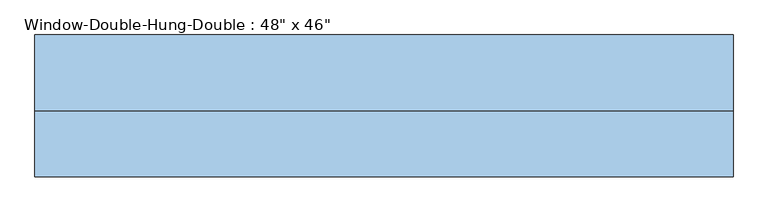
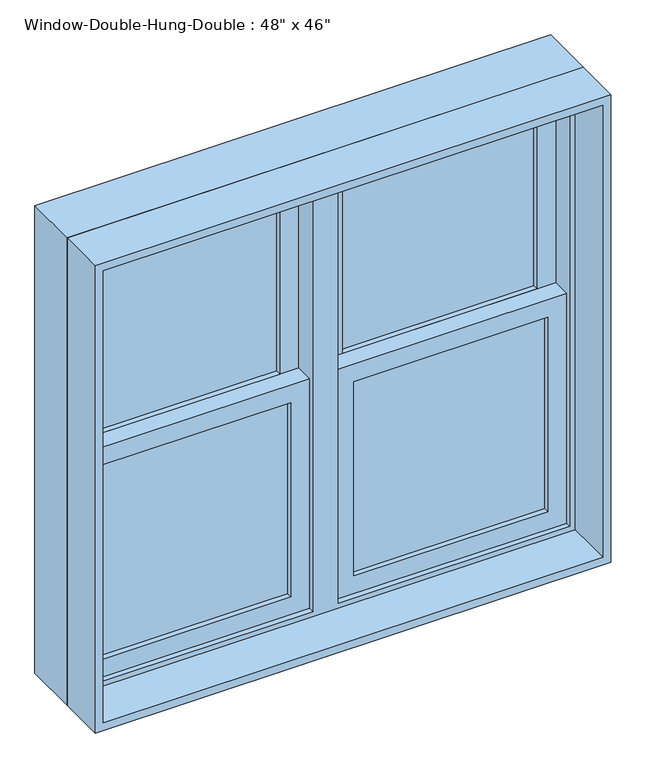
"""IFC4 building model written with IfcOpenShell, lengths in millimetres: window geometry."""

from ifc_helpers import new_model, si_unit, frame, origin, place, context, project, spatial, polyline, outline, extrude, source, transform, mapped, element, save


def window_e23adcbe(model_context):
    return source(origin(), model_context, "Body", "SweptSolid", [
        extrude(outline(polyline([(2082.8, 609.6), (2082.8, -609.6), (914.4, -609.6), (914.4, 609.6), (2082.8, 609.6)]), holes=[polyline([(2063.75, 590.55), (933.45, 590.55), (933.45, -590.55), (2063.75, -590.55), (2063.75, 590.55)])]), frame((0.0, -114.3, 0.0), z_axis=(0.0, 1.0, 0.0), x_axis=(0.0, 0.0, 1.0)), (0.0, 0.0, 1.0), 114.3),
        extrude(outline(polyline([(2051.05, 30.1625), (1476.375, 30.1625), (1476.375, 577.85), (2051.05, 577.85), (2051.05, 30.1625)]), holes=[polyline([(2006.6, 533.4), (1520.825, 533.4), (1520.825, 74.6125), (2006.6, 74.6125), (2006.6, 533.4)])]), frame((0.0, 57.15, 0.0), z_axis=(0.0, 1.0, 0.0), x_axis=(0.0, 0.0, 1.0)), (0.0, 0.0, 1.0), 44.45),
        extrude(outline(polyline([(1520.825, 30.1625), (946.15, 30.1625), (946.15, 577.85), (1520.825, 577.85), (1520.825, 30.1625)]), holes=[polyline([(1476.375, 533.4), (990.6, 533.4), (990.6, 74.6125), (1476.375, 74.6125), (1476.375, 533.4)])]), frame((0.0, 12.7, 0.0), z_axis=(0.0, 1.0, 0.0), x_axis=(0.0, 0.0, 1.0)), (0.0, 0.0, 1.0), 44.45),
        extrude(outline(polyline([(533.4, 88.9), (533.4, 82.55), (74.6125, 82.55), (74.6125, 88.9), (533.4, 88.9)])), frame((0.0, 0.0, 1520.825), z_axis=(0.0, 0.0, 1.0), x_axis=(1.0, 0.0, 0.0)), (0.0, 0.0, 1.0), 485.775),
        extrude(outline(polyline([(74.6125, 76.2), (533.4, 76.2), (533.4, 69.85), (74.6125, 69.85), (74.6125, 76.2)])), frame((0.0, 0.0, 1520.825), z_axis=(0.0, 0.0, 1.0), x_axis=(1.0, 0.0, 0.0)), (0.0, 0.0, 1.0), 485.775),
        extrude(outline(polyline([(533.4, 44.45), (533.4, 38.1), (74.6125, 38.1), (74.6125, 44.45), (533.4, 44.45)])), frame((0.0, 0.0, 990.6), z_axis=(0.0, 0.0, 1.0), x_axis=(1.0, 0.0, 0.0)), (0.0, 0.0, 1.0), 485.775),
        extrude(outline(polyline([(74.6125, 31.75), (533.4, 31.75), (533.4, 25.4), (74.6125, 25.4), (74.6125, 31.75)])), frame((0.0, 0.0, 990.6), z_axis=(0.0, 0.0, 1.0), x_axis=(1.0, 0.0, 0.0)), (0.0, 0.0, 1.0), 485.775),
        extrude(outline(polyline([(2051.05, -577.85), (1476.375, -577.85), (1476.375, -30.1625), (2051.05, -30.1625), (2051.05, -577.85)]), holes=[polyline([(2006.6, -74.6125), (1520.825, -74.6125), (1520.825, -533.4), (2006.6, -533.4), (2006.6, -74.6125)])]), frame((0.0, 57.15, 0.0), z_axis=(0.0, 1.0, 0.0), x_axis=(0.0, 0.0, 1.0)), (0.0, 0.0, 1.0), 44.45),
        extrude(outline(polyline([(1520.825, -577.85), (946.15, -577.85), (946.15, -30.1625), (1520.825, -30.1625), (1520.825, -577.85)]), holes=[polyline([(1476.375, -74.6125), (990.6, -74.6125), (990.6, -533.4), (1476.375, -533.4), (1476.375, -74.6125)])]), frame((0.0, 12.7, 0.0), z_axis=(0.0, 1.0, 0.0), x_axis=(0.0, 0.0, 1.0)), (0.0, 0.0, 1.0), 44.45),
        extrude(outline(polyline([(-533.4, 88.9), (-74.6125, 88.9), (-74.6125, 82.55), (-533.4, 82.55), (-533.4, 88.9)])), frame((0.0, 0.0, 1520.825), z_axis=(0.0, 0.0, 1.0), x_axis=(1.0, 0.0, 0.0)), (0.0, 0.0, 1.0), 485.775),
        extrude(outline(polyline([(-74.6125, 76.2), (-74.6125, 69.85), (-533.4, 69.85), (-533.4, 76.2), (-74.6125, 76.2)])), frame((0.0, 0.0, 1520.825), z_axis=(0.0, 0.0, 1.0), x_axis=(1.0, 0.0, 0.0)), (0.0, 0.0, 1.0), 485.775),
        extrude(outline(polyline([(-533.4, 44.45), (-74.6125, 44.45), (-74.6125, 38.1), (-533.4, 38.1), (-533.4, 44.45)])), frame((0.0, 0.0, 990.6), z_axis=(0.0, 0.0, 1.0), x_axis=(1.0, 0.0, 0.0)), (0.0, 0.0, 1.0), 485.775),
        extrude(outline(polyline([(-74.6125, 31.75), (-74.6125, 25.4), (-533.4, 25.4), (-533.4, 31.75), (-74.6125, 31.75)])), frame((0.0, 0.0, 990.6), z_axis=(0.0, 0.0, 1.0), x_axis=(1.0, 0.0, 0.0)), (0.0, 0.0, 1.0), 485.775),
        extrude(outline(polyline([(2082.8, 609.6), (2082.8, -609.6), (914.4, -609.6), (914.4, 609.6), (2082.8, 609.6)]), holes=[polyline([(946.15, -577.85), (2051.05, -577.85), (2051.05, -30.1625), (946.15, -30.1625), (946.15, -577.85)]), polyline([(946.15, 577.85), (946.15, 30.1625), (2051.05, 30.1625), (2051.05, 577.85), (946.15, 577.85)])]), frame((0.0, 0.0, 0.0), z_axis=(0.0, 1.0, 0.0), x_axis=(0.0, 0.0, 1.0)), (0.0, 0.0, 1.0), 133.35),
    ])


if __name__ == "__main__":
    model = new_model("IFC4")
    model_context = context("Model", 3, world=origin())
    ifc_project = project(units=[si_unit("LENGTHUNIT", "METRE", prefix="MILLI")], contexts=[model_context])
    site = spatial("IfcSite", under=ifc_project)
    building = spatial("IfcBuilding", under=site)
    placement = place(None, origin())
    window_shape = window_e23adcbe(model_context)
    element("IfcWindow", 1, ObjectType="Window-Double-Hung-Double : 48\" x 46\"", at=placement, inside=building, context=model_context, shape_type="MappedRepresentation", body=[
        mapped(window_shape, transform((0.0, 0.0, 0.0), x_axis=(1.0, 0.0, 0.0), y_axis=(0.0, 1.0, 0.0), z_axis=(0.0, 0.0, 1.0))),
    ])
    save(model, "model.ifc")

# Revit data of these elements
# Type "Window-Double-Hung-Double : 48\" x 46\""
#   Type Mark = "21"
#   Fire Rating = "0.5h"
#   Construction Type Id = "DG-DR"
#   Assembly Code = "B2020100"
#   Analytic Construction = "Double glazing - domestic"
#   Wall Thickness [instance default] = 0' - 6"
#   Window Inset [instance default] = 0' - 0"
#   Visual Light Transmittance = 0.81
#   Thermal Resistance (R) = 1.8146 (h·ft²·°F)/BTU
#   Solar Heat Gain Coefficient = 0.76
#   Muntin Width = 1' - 6 1/16"
#   Muntin Height = 1' - 7 1/8"
#   Interior Wall Closure [instance default] = 0' - 1 1/2"
#   Rough Width = 4' - 0 1/2"
#   Rough Height = 3' - 10 1/2"
#   Frame Extension [instance default] = 0' - 1 1/4"
#   Exterior Wall Closure [instance default] = 0' - 0 1/2"
#   Extension Jamb [instance default] = 0' - 1 1/2"
#   Heat Transfer Coefficient (U) = 0.5511 BTU/(h·ft²·°F)
#   Height = 3' - 10"
#   Width = 4' - 0"
#   Top Muntin Visibility = yes
#   Indicator Visibility [instance default] = yes
#   Extension Jamb Visibility [instance default] = yes
#   Interior Trim Visibility [instance default] = yes
#   Exterior Trim Visibility [instance default] = yes
#   Define Thermal Properties by = 1
#   Bottom Muntin Visibility = yes
#   Muntin Pattern = Muntin Pattern_2x2 : Muntin Pattern_2x2
#   Interior Trim Material = Wood - Stained
#   Interior Trim = Trim-Window-Interior-Flat : Picture Frame
#   Exterior Trim Material = Clad - White
#   Exterior Trim = Trim-Window-Exterior-Flat : with Sill
#   Glass Panel Material = Glass
#   Exterior Frame Material = Clad - White
#   Interior Frame Material = Wood - Stained
#   Wall Closure = (empty or 0)
# Element 1 (IfcWindow, "Window-Double-Hung-Double : 48\" x 46\"")
#   Wall Thickness = 0' - 9"
#   Extension Jamb = 0' - 4 1/2"
#   Materials on its faces: "Wood - Stained", "Glass", "Clad - White"
# Materials
#   "Wood - Stained": class "Wood", colour RGB 224 178 126, transparency 0, Cost = 0
#   "Clad - White": class "Wood", colour RGB 242 242 238, transparency 0, Cost = 0
#   "Glass": class "Glass", colour RGB 0 128 192, transparency 0.75, Description = "Soda Lime Glass", Cost = 0
